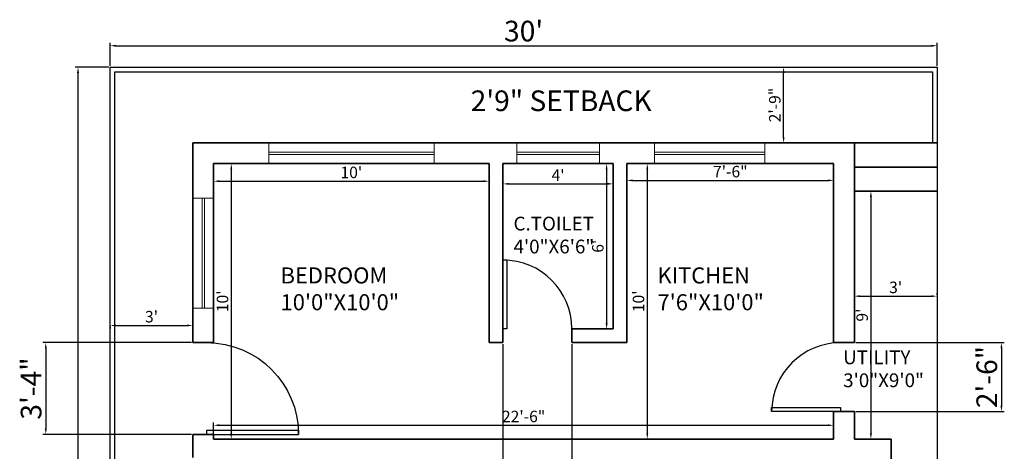
# Model space of a CAD drawing. Units: inches. Extents: x 2831 to 4250, y 1103 to 1797.
# Tile 15 of 15: x 3821 to 4250, y 1555 to 1743. Entities that reach past the tile are written whole.
import ezdxf

# ---------------------------------------------------------------- set-up
doc = ezdxf.new("R2010")
doc.units = ezdxf.units.IN
for name, color, linetype, lineweight in [('A-ANNO-DIMS', 2, 'Continuous', 18), ('A-ANNO-TEXT', 7, 'Continuous', 18), ('A-AREA-IDEN', 7, 'Continuous', 18), ('A-DOOR', 4, 'Continuous', 25), ('A-WALL', 7, 'Continuous', 35), ('C-PROP', 7, 'Continuous', 25), ('window', 130, 'Continuous', 18)]:
    doc.layers.add(name, color=color, linetype=linetype, lineweight=lineweight)
doc.styles.get("Standard").update_dxf_attribs({"font": 'arial.ttf'})
doc.dimstyles.new('ISO-25', dxfattribs={"dimtxt": 9, "dimasz": 2.5, "dimexe": 1.25, "dimexo": 0.625, "dimtad": 1, "dimdec": 1, "dimlunit": 3, "dimtxsty": 'Standard', "dimcen": 2.5, "dimadec": 0, "dimazin": 0, "dimtfac": 1, "dimtdec": 1, "dimtmove": 0, "dimatfit": 3, "dimfxl": 1, "dimarcsym": 0})

# ---------------------------------------------------------------- blocks, each defined once
blk = doc.blocks.new('*U2')
for p, q in [((0, 0), (0, -6)), ((40, 0), (40, -6))]:
    blk.add_line(p, q)
blk.add_lwpolyline([(0, 0), (0, 40), (1.75, 40), (1.75, 0)], close=True)
blk.add_arc((0, 0), 40, 0, 90)
blk = doc.blocks.new('*U4')
for p, q in [((0, 0), (0, -6)), ((30, 0), (30, -6))]:
    blk.add_line(p, q)
blk.add_lwpolyline([(0, 0), (0, 30), (1.75, 30), (1.75, 0)], close=True)
blk.add_arc((0, 0), 30, 0, 90)
blk = doc.blocks.new('*D28')
at = {"layer": 'A-ANNO-DIMS', "color": 0, "lineweight": -2, "transparency": 16777216}
for p, q in [((3860.39, 1723.14), (3860.39, 1733.1)), ((4220.39, 1723.14), (4220.39, 1733.1)), ((3862.89, 1731.85), (4217.89, 1731.85))]:
    blk.add_line(p, q, dxfattribs=at)
at = {"layer": 'A-ANNO-DIMS', "color": 0, "transparency": 16777216}
for points in [[(3862.89, 1732.27), (3862.89, 1731.43), (3860.39, 1731.85)], [(4217.89, 1732.27), (4217.89, 1731.43), (4220.39, 1731.85)]]:
    blk.add_solid(points, dxfattribs=at)
at = {"layer": 'Defpoints', "color": 0, "transparency": 16777216}
for p in [(4220.39, 1731.85), (3860.39, 1722.51), (4220.39, 1722.51)]:
    blk.add_point(p, dxfattribs=at)
at = {"layer": 'A-ANNO-DIMS', "color": 0, "transparency": 16777216, "insert": (4040.39, 1737.07), "char_height": 9, "attachment_point": 5}
blk.add_mtext("30'", dxfattribs=at)
blk = doc.blocks.new('*D29')
at = {"layer": 'A-ANNO-DIMS', "color": 0, "lineweight": -2, "transparency": 16777216}
for p, q in [((3859.76, 1722.51), (3845.12, 1722.51)), ((3846.37, 1720.01), (3846.37, 1245.01)), ((3859.76, 1242.51), (3845.12, 1242.51))]:
    blk.add_line(p, q, dxfattribs=at)
at = {"layer": 'A-ANNO-DIMS', "color": 0, "transparency": 16777216}
for points in [[(3845.95, 1720.01), (3846.79, 1720.01), (3846.37, 1722.51)], [(3845.95, 1245.01), (3846.79, 1245.01), (3846.37, 1242.51)]]:
    blk.add_solid(points, dxfattribs=at)
at = {"layer": 'Defpoints', "color": 0, "transparency": 16777216}
for p in [(3860.39, 1722.51), (3846.37, 1242.51), (3860.39, 1242.51)]:
    blk.add_point(p, dxfattribs=at)
at = {"layer": 'A-ANNO-DIMS', "color": 0, "transparency": 16777216, "insert": (3841.15, 1482.51), "char_height": 9, "attachment_point": 5, "rotation": 90}
blk.add_mtext("40'", dxfattribs=at)
blk = doc.blocks.new('*D30')
at = {"layer": 'A-ANNO-DIMS', "color": 0, "lineweight": -2, "transparency": 16777216}
for p, q in [((3905.39, 1679.89), (3905.39, 1671.58)), ((4025.39, 1679.89), (4025.39, 1671.58)), ((3907.89, 1672.83), (4022.89, 1672.83))]:
    blk.add_line(p, q, dxfattribs=at)
at = {"layer": 'A-ANNO-DIMS', "color": 0, "transparency": 16777216}
for points in [[(3907.89, 1673.25), (3907.89, 1672.42), (3905.39, 1672.83)], [(4022.89, 1673.25), (4022.89, 1672.42), (4025.39, 1672.83)]]:
    blk.add_solid(points, dxfattribs=at)
at = {"layer": 'Defpoints', "color": 0, "transparency": 16777216}
for p in [(3905.39, 1680.51), (4025.39, 1680.51), (4025.39, 1672.83)]:
    blk.add_point(p, dxfattribs=at)
at = {"layer": 'A-ANNO-DIMS', "color": 0, "transparency": 16777216, "insert": (3965.39, 1676.01), "char_height": 5, "attachment_point": 5}
blk.add_mtext("10'", dxfattribs=at)
blk = doc.blocks.new('*D31')
at = {"layer": 'A-ANNO-DIMS', "color": 0, "lineweight": -2, "transparency": 16777216}
for p, q in [((3906.01, 1680.51), (3914.36, 1680.51)), ((3913.11, 1678.01), (3913.11, 1563.01)), ((3906.01, 1560.51), (3914.36, 1560.51))]:
    blk.add_line(p, q, dxfattribs=at)
at = {"layer": 'A-ANNO-DIMS', "color": 0, "transparency": 16777216}
for points in [[(3912.7, 1678.01), (3913.53, 1678.01), (3913.11, 1680.51)], [(3912.7, 1563.01), (3913.53, 1563.01), (3913.11, 1560.51)]]:
    blk.add_solid(points, dxfattribs=at)
at = {"layer": 'Defpoints', "color": 0, "transparency": 16777216}
for p in [(3905.39, 1680.51), (3905.39, 1560.51), (3913.11, 1560.51)]:
    blk.add_point(p, dxfattribs=at)
at = {"layer": 'A-ANNO-DIMS', "color": 0, "transparency": 16777216, "insert": (3909.94, 1620.51), "char_height": 5, "attachment_point": 5, "rotation": 90}
blk.add_mtext("10'", dxfattribs=at)
blk = doc.blocks.new('*D32')
at = {"layer": 'A-ANNO-DIMS', "color": 0, "lineweight": -2, "transparency": 16777216}
for p, q in [((4031.39, 1679.89), (4031.39, 1670.42)), ((4079.39, 1679.89), (4079.39, 1670.42)), ((4033.89, 1671.67), (4076.89, 1671.67))]:
    blk.add_line(p, q, dxfattribs=at)
at = {"layer": 'A-ANNO-DIMS', "color": 0, "transparency": 16777216}
for points in [[(4033.89, 1672.09), (4033.89, 1671.26), (4031.39, 1671.67)], [(4076.89, 1672.09), (4076.89, 1671.26), (4079.39, 1671.67)]]:
    blk.add_solid(points, dxfattribs=at)
at = {"layer": 'Defpoints', "color": 0, "transparency": 16777216}
for p in [(4031.39, 1680.51), (4079.39, 1680.51), (4079.39, 1671.67)]:
    blk.add_point(p, dxfattribs=at)
at = {"layer": 'A-ANNO-DIMS', "color": 0, "transparency": 16777216, "insert": (4055.39, 1674.8), "char_height": 5, "attachment_point": 5}
blk.add_mtext("4'", dxfattribs=at)
blk = doc.blocks.new('*D33')
at = {"layer": 'A-ANNO-DIMS', "color": 0, "lineweight": -2, "transparency": 16777216}
for p, q in [((4078.76, 1680.51), (4075.28, 1680.51)), ((4076.53, 1678.01), (4076.53, 1611.01)), ((4078.76, 1608.51), (4075.28, 1608.51))]:
    blk.add_line(p, q, dxfattribs=at)
at = {"layer": 'A-ANNO-DIMS', "color": 0, "transparency": 16777216}
for points in [[(4076.11, 1678.01), (4076.95, 1678.01), (4076.53, 1680.51)], [(4076.11, 1611.01), (4076.95, 1611.01), (4076.53, 1608.51)]]:
    blk.add_solid(points, dxfattribs=at)
at = {"layer": 'Defpoints', "color": 0, "transparency": 16777216}
for p in [(4079.39, 1680.51), (4076.53, 1608.51), (4079.39, 1608.51)]:
    blk.add_point(p, dxfattribs=at)
at = {"layer": 'A-ANNO-DIMS', "color": 0, "transparency": 16777216, "insert": (4073.35, 1644.51), "char_height": 5, "attachment_point": 5, "rotation": 90}
blk.add_mtext("6'", dxfattribs=at)
blk = doc.blocks.new('*D34')
at = {"layer": 'A-ANNO-DIMS', "color": 0, "lineweight": -2, "transparency": 16777216}
for p, q in [((4085.39, 1679.89), (4085.39, 1671.93)), ((4175.39, 1679.89), (4175.39, 1671.93)), ((4087.89, 1673.18), (4172.89, 1673.18))]:
    blk.add_line(p, q, dxfattribs=at)
at = {"layer": 'A-ANNO-DIMS', "color": 0, "transparency": 16777216}
for points in [[(4087.89, 1673.6), (4087.89, 1672.76), (4085.39, 1673.18)], [(4172.89, 1673.6), (4172.89, 1672.76), (4175.39, 1673.18)]]:
    blk.add_solid(points, dxfattribs=at)
at = {"layer": 'Defpoints', "color": 0, "transparency": 16777216}
for p in [(4085.39, 1680.51), (4175.39, 1680.51), (4175.39, 1673.18)]:
    blk.add_point(p, dxfattribs=at)
at = {"layer": 'A-ANNO-DIMS', "color": 0, "transparency": 16777216, "insert": (4130.39, 1676.36), "char_height": 5, "attachment_point": 5}
blk.add_mtext('7\'-6"', dxfattribs=at)
blk = doc.blocks.new('*D35')
at = {"layer": 'A-ANNO-DIMS', "color": 0, "lineweight": -2, "transparency": 16777216}
for p, q in [((4086.01, 1680.51), (4095.49, 1680.51)), ((4094.24, 1678.01), (4094.24, 1563.01)), ((4086.01, 1560.51), (4095.49, 1560.51))]:
    blk.add_line(p, q, dxfattribs=at)
at = {"layer": 'A-ANNO-DIMS', "color": 0, "transparency": 16777216}
for points in [[(4093.82, 1678.01), (4094.66, 1678.01), (4094.24, 1680.51)], [(4093.82, 1563.01), (4094.66, 1563.01), (4094.24, 1560.51)]]:
    blk.add_solid(points, dxfattribs=at)
at = {"layer": 'Defpoints', "color": 0, "transparency": 16777216}
for p in [(4085.39, 1680.51), (4085.39, 1560.51), (4094.24, 1560.51)]:
    blk.add_point(p, dxfattribs=at)
at = {"layer": 'A-ANNO-DIMS', "color": 0, "transparency": 16777216, "insert": (4091.06, 1620.51), "char_height": 5, "attachment_point": 5, "rotation": 90}
blk.add_mtext("10'", dxfattribs=at)
blk = doc.blocks.new('*D36')
at = {"layer": 'A-ANNO-DIMS', "color": 0, "lineweight": -2, "transparency": 16777216}
for p, q in [((4184.39, 1623.37), (4184.39, 1624)), ((4186.89, 1622.75), (4217.89, 1622.75)), ((4220.39, 1623.37), (4220.39, 1624))]:
    blk.add_line(p, q, dxfattribs=at)
at = {"layer": 'A-ANNO-DIMS', "color": 0, "transparency": 16777216}
for points in [[(4186.89, 1623.16), (4186.89, 1622.33), (4184.39, 1622.75)], [(4217.89, 1623.16), (4217.89, 1622.33), (4220.39, 1622.75)]]:
    blk.add_solid(points, dxfattribs=at)
at = {"layer": 'Defpoints', "color": 0, "transparency": 16777216}
for p in [(4184.39, 1622.75), (4220.39, 1622.75), (4220.39, 1622.75)]:
    blk.add_point(p, dxfattribs=at)
at = {"layer": 'A-ANNO-DIMS', "color": 0, "transparency": 16777216, "insert": (4202.39, 1625.93), "char_height": 5, "attachment_point": 5}
blk.add_mtext("3'", dxfattribs=at)
blk = doc.blocks.new('*D37')
at = {"layer": 'A-ANNO-DIMS', "color": 0, "lineweight": -2, "transparency": 16777216}
for p, q in [((4193.23, 1668.51), (4190.36, 1668.51)), ((4191.61, 1666.01), (4191.61, 1563.01)), ((4191.76, 1560.51), (4190.36, 1560.51))]:
    blk.add_line(p, q, dxfattribs=at)
at = {"layer": 'A-ANNO-DIMS', "color": 0, "transparency": 16777216}
for points in [[(4191.19, 1666.01), (4192.03, 1666.01), (4191.61, 1668.51)], [(4191.19, 1563.01), (4192.03, 1563.01), (4191.61, 1560.51)]]:
    blk.add_solid(points, dxfattribs=at)
at = {"layer": 'Defpoints', "color": 0, "transparency": 16777216}
for p in [(4193.86, 1668.51), (4191.61, 1560.51), (4192.39, 1560.51)]:
    blk.add_point(p, dxfattribs=at)
at = {"layer": 'A-ANNO-DIMS', "color": 0, "transparency": 16777216, "insert": (4188.43, 1614.51), "char_height": 5, "attachment_point": 5, "rotation": 90}
blk.add_mtext("9'", dxfattribs=at)
blk = doc.blocks.new('*D38')
at = {"layer": 'A-ANNO-DIMS', "color": 0, "lineweight": -2, "transparency": 16777216}
for p, q in [((3905.39, 1561.14), (3905.39, 1567.76)), ((3907.89, 1566.51), (4172.89, 1566.51)), ((4175.39, 1561.14), (4175.39, 1567.76))]:
    blk.add_line(p, q, dxfattribs=at)
at = {"layer": 'A-ANNO-DIMS', "color": 0, "transparency": 16777216}
for points in [[(3907.89, 1566.93), (3907.89, 1566.1), (3905.39, 1566.51)], [(4172.89, 1566.93), (4172.89, 1566.1), (4175.39, 1566.51)]]:
    blk.add_solid(points, dxfattribs=at)
at = {"layer": 'Defpoints', "color": 0, "transparency": 16777216}
for p in [(4175.39, 1566.51), (3905.39, 1560.51), (4175.39, 1560.51)]:
    blk.add_point(p, dxfattribs=at)
at = {"layer": 'A-ANNO-DIMS', "color": 0, "transparency": 16777216, "insert": (4040.39, 1569.69), "char_height": 5, "attachment_point": 5}
blk.add_mtext('22\'-6"', dxfattribs=at)
blk = doc.blocks.new('*D65')
at = {"layer": 'A-ANNO-DIMS', "color": 0, "lineweight": -2, "transparency": 16777216}
for p, q in [((4153.59, 1692.01), (4153.59, 1720.01)), ((4154.22, 1722.51), (4154.84, 1722.51)), ((4154.22, 1689.51), (4154.84, 1689.51))]:
    blk.add_line(p, q, dxfattribs=at)
at = {"layer": 'A-ANNO-DIMS', "color": 0, "transparency": 16777216}
for points in [[(4153.18, 1720.01), (4154.01, 1720.01), (4153.59, 1722.51)], [(4153.18, 1692.01), (4154.01, 1692.01), (4153.59, 1689.51)]]:
    blk.add_solid(points, dxfattribs=at)
at = {"layer": 'Defpoints', "color": 0, "transparency": 16777216}
for p in [(4153.59, 1722.51), (4153.59, 1722.51), (4153.59, 1689.51)]:
    blk.add_point(p, dxfattribs=at)
at = {"layer": 'A-ANNO-DIMS', "color": 0, "transparency": 16777216, "insert": (4150.42, 1706.01), "char_height": 5, "attachment_point": 5, "rotation": 90}
blk.add_mtext('2\'-9"', dxfattribs=at)
blk = doc.blocks.new('*D66')
at = {"layer": 'A-ANNO-DIMS', "color": 0, "lineweight": -2, "transparency": 16777216}
for p, q in [((3860.39, 1609.36), (3860.39, 1608.73)), ((3862.89, 1609.98), (3893.89, 1609.98)), ((3896.39, 1610.61), (3896.39, 1611.23))]:
    blk.add_line(p, q, dxfattribs=at)
at = {"layer": 'A-ANNO-DIMS', "color": 0, "transparency": 16777216}
for points in [[(3862.89, 1610.4), (3862.89, 1609.57), (3860.39, 1609.98)], [(3893.89, 1610.4), (3893.89, 1609.57), (3896.39, 1609.98)]]:
    blk.add_solid(points, dxfattribs=at)
at = {"layer": 'Defpoints', "color": 0, "transparency": 16777216}
for p in [(3860.39, 1609.98), (3896.39, 1609.98), (3896.39, 1609.98)]:
    blk.add_point(p, dxfattribs=at)
at = {"layer": 'A-ANNO-DIMS', "color": 0, "transparency": 16777216, "insert": (3878.39, 1613.16), "char_height": 5, "attachment_point": 5}
blk.add_mtext("3'", dxfattribs=at)
blk = doc.blocks.new('WIN-36IN')
for p, q in [((0, 36), (9, 36)), ((4, 0), (4, 36)), ((5, 0), (5, 36)), ((0, 0), (9, 0))]:
    blk.add_line(p, q)
blk = doc.blocks.new('WIN-48IN')
for p, q in [((9, 48), (0, 48)), ((4, 0), (4, 48)), ((5, 0), (5, 48)), ((9, 0), (0, 0))]:
    blk.add_line(p, q)
blk = doc.blocks.new('WIN-72IN')
for p, q in [((0, 0), (0, 9)), ((72, 0), (72, 9)), ((0, 5), (72, 5)), ((0, 4), (72, 4))]:
    blk.add_line(p, q)
blk = doc.blocks.new('*D99')
at = {"layer": 'A-ANNO-DIMS', "color": 0, "lineweight": -2, "transparency": 16777216}
for p, q in [((3895.76, 1602.51), (3831.09, 1602.51)), ((3832.34, 1600.01), (3832.34, 1565.01)), ((3895.76, 1562.51), (3831.09, 1562.51))]:
    blk.add_line(p, q, dxfattribs=at)
at = {"layer": 'A-ANNO-DIMS', "color": 0, "transparency": 16777216}
for points in [[(3831.92, 1600.01), (3832.76, 1600.01), (3832.34, 1602.51)], [(3831.92, 1565.01), (3832.76, 1565.01), (3832.34, 1562.51)]]:
    blk.add_solid(points, dxfattribs=at)
at = {"layer": 'Defpoints', "color": 0, "transparency": 16777216}
for p in [(3896.39, 1602.51), (3832.34, 1562.51), (3896.39, 1562.51)]:
    blk.add_point(p, dxfattribs=at)
at = {"layer": 'A-ANNO-DIMS', "color": 0, "transparency": 16777216, "insert": (3827.12, 1582.51), "char_height": 9, "attachment_point": 5, "rotation": 90}
blk.add_mtext('3\'-4"', dxfattribs=at)
blk = doc.blocks.new('*D101')
at = {"layer": 'A-ANNO-DIMS', "color": 0, "lineweight": -2, "transparency": 16777216}
for p, q in [((4031.39, 1601.89), (4031.39, 1181)), ((4061.39, 1601.89), (4061.39, 1181)), ((4033.89, 1182.25), (4058.89, 1182.25))]:
    blk.add_line(p, q, dxfattribs=at)
at = {"layer": 'A-ANNO-DIMS', "color": 0, "transparency": 16777216}
for points in [[(4033.89, 1182.67), (4033.89, 1181.83), (4031.39, 1182.25)], [(4058.89, 1182.67), (4058.89, 1181.83), (4061.39, 1182.25)]]:
    blk.add_solid(points, dxfattribs=at)
at = {"layer": 'Defpoints', "color": 0, "transparency": 16777216}
for p in [(4031.39, 1602.51), (4061.39, 1602.51), (4061.39, 1182.25)]:
    blk.add_point(p, dxfattribs=at)
at = {"layer": 'A-ANNO-DIMS', "color": 0, "transparency": 16777216, "insert": (4046.39, 1187.47), "char_height": 9, "attachment_point": 5}
blk.add_mtext('2\'-6"', dxfattribs=at)
blk = doc.blocks.new('*D102')
at = {"layer": 'A-ANNO-DIMS', "color": 0, "lineweight": -2, "transparency": 16777216}
for p, q in [((4185.01, 1602.51), (4249.69, 1602.51)), ((4248.44, 1600.01), (4248.44, 1575.01)), ((4185.01, 1572.51), (4249.69, 1572.51))]:
    blk.add_line(p, q, dxfattribs=at)
at = {"layer": 'A-ANNO-DIMS', "color": 0, "transparency": 16777216}
for points in [[(4248.02, 1600.01), (4248.86, 1600.01), (4248.44, 1602.51)], [(4248.02, 1575.01), (4248.86, 1575.01), (4248.44, 1572.51)]]:
    blk.add_solid(points, dxfattribs=at)
at = {"layer": 'Defpoints', "color": 0, "transparency": 16777216}
for p in [(4184.39, 1602.51), (4184.39, 1572.51), (4248.44, 1572.51)]:
    blk.add_point(p, dxfattribs=at)
at = {"layer": 'A-ANNO-DIMS', "color": 0, "transparency": 16777216, "insert": (4243.22, 1587.51), "char_height": 9, "attachment_point": 5, "rotation": 90}
blk.add_mtext('2\'-6"', dxfattribs=at)

msp = doc.modelspace()

# ---------------------------------------------------------------- linework, layer by layer
at = {"layer": 'A-WALL'}
for p, q in [((3896.39, 1689.51), (4220.39, 1689.51)), ((3896.39, 1602.51), (3896.39, 1689.51)), ((4184.39, 1689.51), (4184.39, 1602.51)), ((3905.39, 1680.51), (4025.39, 1680.51)), ((3905.39, 1602.51), (3905.39, 1680.51)), ((4025.39, 1602.51), (4025.39, 1680.51)), ((4031.39, 1680.51), (4079.39, 1680.51)), ((4031.39, 1602.51), (4031.39, 1680.51)), ((4079.39, 1608.51), (4079.39, 1680.51)), ((4085.39, 1680.51), (4175.39, 1680.51)), ((4085.39, 1602.51), (4085.39, 1680.51)), ((4175.39, 1680.51), (4175.39, 1602.51)), ((4184.39, 1679.01), (4220.39, 1679.01)), ((4184.39, 1668.51), (4220.39, 1668.51)), ((4061.39, 1608.51), (4079.39, 1608.51)), ((4061.39, 1602.51), (4061.39, 1608.51)), ((3896.39, 1602.51), (3905.39, 1602.51)), ((4025.39, 1602.51), (4031.39, 1602.51)), ((4061.39, 1602.51), (4085.39, 1602.51)), ((4175.39, 1602.51), (4184.39, 1602.51)), ((4175.39, 1572.51), (4184.39, 1572.51)), ((4175.39, 1572.51), (4175.39, 1560.51)), ((4184.39, 1572.51), (4184.39, 1560.51)), ((3896.39, 1562.51), (3905.39, 1562.51)), ((3896.39, 1552.51), (3896.39, 1562.51)), ((3905.39, 1560.51), (3905.39, 1562.51)), ((3905.39, 1560.51), (4175.39, 1560.51)), ((4184.39, 1560.51), (4200.39, 1560.51)), ((4200.39, 1460.51), (4200.39, 1560.51))]:
    msp.add_line(p, q, dxfattribs=at)
at = {"layer": 'C-PROP'}
msp.add_line((4218.39, 1720.51), (4218.39, 1689.51), dxfattribs=at)
msp.add_lwpolyline([(3860.39, 1722.51), (4220.39, 1722.51), (4220.39, 1242.51), (3860.39, 1242.51)], close=True, dxfattribs=at)
msp.add_lwpolyline([(3862.39, 1244.51), (3862.39, 1720.51), (4218.39, 1720.51)], dxfattribs=at)

# ---------------------------------------------------------------- block references
at = {"layer": 'A-DOOR'}
msp.add_blockref('*U4', (4031.39, 1608.51), dxfattribs=at)
at = {"layer": 'A-DOOR', "xscale": -1, "rotation": 270}
msp.add_blockref('*U2', (3902.39, 1562.51), dxfattribs=at)
at = {"layer": 'A-DOOR', "rotation": 90}
msp.add_blockref('*U4', (4178.39, 1572.51), dxfattribs=at)
at = {"layer": 'window'}
for name, p, rotation in [('WIN-72IN', (4001.39, 1689.51), 180), ('WIN-36IN', (4073.39, 1680.51), 89.99999999999557), ('WIN-48IN', (4145.39, 1680.51), 90)]:
    msp.add_blockref(name, p, dxfattribs=dict(at, rotation=rotation))
msp.add_blockref('WIN-48IN', (3896.39, 1617.51), dxfattribs=at)

# ---------------------------------------------------------------- texts
at = {"layer": 'A-ANNO-TEXT', "insert": (4017.33, 1712.37), "char_height": 9, "attachment_point": 1}
msp.add_mtext_dynamic_manual_height_columns('{\\fTimes New Roman|b0|i0|c0|p18;2\'9" SETBACK}', width=97.569, gutter_width=12.5, heights=[0], dxfattribs=at)
at = {"layer": 'A-AREA-IDEN', "attachment_point": 1}
for s, insert, char_height in [('{\\fTimes New Roman|b0|i0|c0|p18;C.TOILET\\P4\'0"X6\'6"}', (4035.99, 1657.37), 6), ('{\\fTimes New Roman|b0|i0|c0|p18;BEDROOM\\P10\'0"X10\'0"}', (3934.57, 1635.28), 7), ('{\\fTimes New Roman|b0|i0|c0|p18;KITCHEN\\P7\'6"X10\'0"}', (4098.68, 1635.28), 7), ('{\\fTimes New Roman|b0|i0|c0|p18;UTILITY\\P3\'0"X9\'0"}', (4179.52, 1599.11), 6)]:
    msp.add_mtext_dynamic_manual_height_columns(s, width=81.5075, gutter_width=12.5, heights=[0], dxfattribs=dict(at, insert=insert, char_height=char_height))

# ---------------------------------------------------------------- dimensions: what is measured, and where the dimension line sits
at = {"layer": 'A-ANNO-DIMS'}
for base, p1, p2, override, picture, middle in [((4220.39, 1731.85), (3860.39, 1722.51), (4220.39, 1722.51), {"dimclrd": 0, "dimclre": 0, "dimclrt": 0}, '*D28', (4040.39, 1737.07)), ((4025.39, 1672.83), (3905.39, 1680.51), (4025.39, 1680.51), {"dimtxt": 5, "dimclrd": 0, "dimclre": 0, "dimclrt": 0}, '*D30', (3965.39, 1676.01)), ((4079.39, 1671.67), (4031.39, 1680.51), (4079.39, 1680.51), {"dimtxt": 5, "dimclrd": 0, "dimclre": 0, "dimclrt": 0}, '*D32', (4055.39, 1674.8)), ((4175.39, 1673.18), (4085.39, 1680.51), (4175.39, 1680.51), {"dimtxt": 5, "dimclrd": 0, "dimclre": 0, "dimclrt": 0}, '*D34', (4130.39, 1676.36)), ((4220.39, 1622.75), (4184.39, 1622.75), (4220.39, 1622.75), {"dimtxt": 5, "dimclrd": 0, "dimclre": 0, "dimclrt": 0}, '*D36', (4202.39, 1625.93)), ((3896.39, 1609.98), (3860.39, 1609.98), (3896.39, 1609.98), {"dimtxt": 5, "dimclrd": 0, "dimclre": 0, "dimclrt": 0}, '*D66', (3878.39, 1613.16)), ((4061.39, 1182.25), (4031.39, 1602.51), (4061.39, 1602.51), {"dimdec": 1, "dimlfac": 1, "dimrnd": 0, "dimzin": 1, "dimdsep": 46, "dimlunit": 4, "dimfrac": 2}, '*D101', (4046.39, 1187.47)), ((4175.39, 1566.51), (3905.39, 1560.51), (4175.39, 1560.51), {"dimtxt": 5, "dimclrd": 0, "dimclre": 0, "dimclrt": 0}, '*D38', (4040.39, 1569.69))]:
    dim = msp.add_linear_dim(base=base, p1=p1, p2=p2, dimstyle='ISO-25', override=override, dxfattribs=at)
    dim.commit()
    dim.dimension.update_dxf_attribs({"geometry": picture, "text_midpoint": middle})
for base, p1, p2, override, picture, middle in [((3846.37, 1242.51), (3860.39, 1722.51), (3860.39, 1242.51), {"dimclrd": 0, "dimclre": 0, "dimclrt": 0}, '*D29', (3841.15, 1482.51)), ((4153.59, 1722.51), (4153.59, 1689.51), (4153.59, 1722.51), {"dimtxt": 5, "dimclrd": 0, "dimclre": 0, "dimclrt": 0}, '*D65', (4150.42, 1706.01)), ((3913.11, 1560.51), (3905.39, 1680.51), (3905.39, 1560.51), {"dimtxt": 5, "dimclrd": 0, "dimclre": 0, "dimclrt": 0}, '*D31', (3909.94, 1620.51)), ((4076.53, 1608.51), (4079.39, 1680.51), (4079.39, 1608.51), {"dimtxt": 5, "dimclrd": 0, "dimclre": 0, "dimclrt": 0}, '*D33', (4073.35, 1644.51)), ((4094.24, 1560.51), (4085.39, 1680.51), (4085.39, 1560.51), {"dimtxt": 5, "dimclrd": 0, "dimclre": 0, "dimclrt": 0}, '*D35', (4091.06, 1620.51)), ((4191.61, 1560.51), (4193.86, 1668.51), (4192.39, 1560.51), {"dimtxt": 5, "dimclrd": 0, "dimclre": 0, "dimclrt": 0}, '*D37', (4188.43, 1614.51)), ((3832.34, 1562.51), (3896.39, 1602.51), (3896.39, 1562.51), {"dimdec": 1, "dimlfac": 1, "dimrnd": 0, "dimzin": 1, "dimdsep": 46, "dimlunit": 4, "dimfrac": 2}, '*D99', (3827.12, 1582.51)), ((4248.44, 1572.51), (4184.39, 1602.51), (4184.39, 1572.51), {"dimdec": 1, "dimlfac": 1, "dimrnd": 0, "dimzin": 1, "dimdsep": 46, "dimlunit": 4, "dimfrac": 2}, '*D102', (4243.22, 1587.51))]:
    dim = msp.add_linear_dim(base=base, p1=p1, p2=p2, angle=90, dimstyle='ISO-25', override=override, dxfattribs=at)
    dim.commit()
    dim.dimension.update_dxf_attribs({"geometry": picture, "text_midpoint": middle})

doc.saveas('drawing.dxf')
